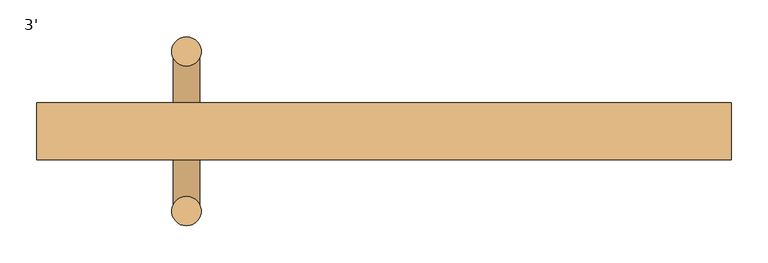
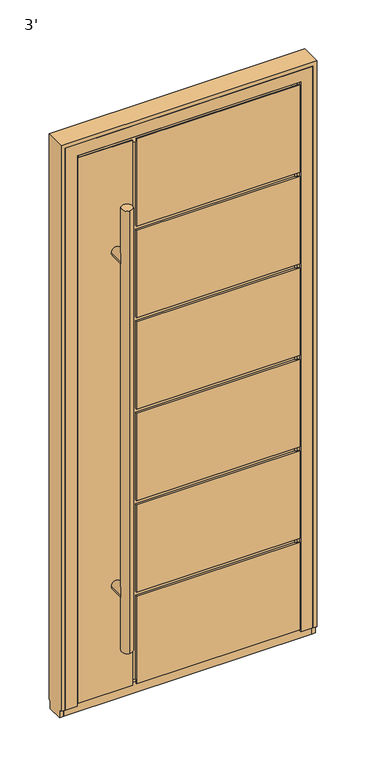
"""IFC4 building model written with IfcOpenShell, lengths in millimetres: door geometry, 3'."""

from ifc_helpers import new_model, si_unit, point, frame, frame_2d, origin, place, context, project, spatial, circle_curve, trimmed, segment, composite_curve, outline, extrude, faceted_brep, source, transform, mapped, element, save


def door_3_79df91aa(model_context):
    return source(origin(), model_context, "Body", "SolidModel", [
        extrude(outline(composite_curve([segment(trimmed(circle_curve(frame_2d((-268.65, 90.8003001)), 20.0), [point((-268.65, 70.8003001))], [point((-268.65, 110.8003001))], False, "CARTESIAN"), True, "CONTINUOUS"), segment(trimmed(circle_curve(frame_2d((-268.65, 90.8003001)), 20.0), [point((-268.65, 110.8003001))], [point((-268.65, 70.8003001))], False, "CARTESIAN"), True, "CONTINUOUS")], self_intersect=False)), frame((0.0, 0.0, 210.0000003), z_axis=(0.0, 0.0, 1.0), x_axis=(1.0, 0.0, 0.0)), (0.0, 0.0, 1.0), 1724.5),
        extrude(outline(composite_curve([segment(trimmed(circle_curve(frame_2d((-268.65, -126.2003001)), 20.0), [point((-268.65, -146.2003001))], [point((-268.65, -106.2003001))], False, "CARTESIAN"), True, "CONTINUOUS"), segment(trimmed(circle_curve(frame_2d((-268.65, -126.2003001)), 20.0), [point((-268.65, -106.2003001))], [point((-268.65, -146.2003001))], False, "CARTESIAN"), True, "CONTINUOUS")], self_intersect=False)), frame((0.0, 0.0, 210.0000003), z_axis=(0.0, 0.0, 1.0), x_axis=(1.0, 0.0, 0.0)), (0.0, 0.0, 1.0), 1724.5),
        extrude(outline(composite_curve([segment(trimmed(circle_curve(frame_2d((422.2500003, -268.65)), 18.0), [point((422.2500003, -286.65))], [point((422.2500003, -250.65))], False, "CARTESIAN"), True, "CONTINUOUS"), segment(trimmed(circle_curve(frame_2d((422.2500003, -268.65)), 18.0), [point((422.2500003, -250.65))], [point((422.2500003, -286.65))], False, "CARTESIAN"), True, "CONTINUOUS")], self_intersect=False)), frame((0.0, -126.2, 0.0), z_axis=(0.0, 1.0, 0.0), x_axis=(0.0, 0.0, 1.0)), (0.0, 0.0, 1.0), 217.0),
        extrude(outline(composite_curve([segment(trimmed(circle_curve(frame_2d((1722.2500003, -268.65)), 18.0), [point((1722.2500003, -286.65))], [point((1722.2500003, -250.65))], False, "CARTESIAN"), True, "CONTINUOUS"), segment(trimmed(circle_curve(frame_2d((1722.2500003, -268.65)), 18.0), [point((1722.2500003, -250.65))], [point((1722.2500003, -286.65))], False, "CARTESIAN"), True, "CONTINUOUS")], self_intersect=False)), frame((0.0, -126.2, 0.0), z_axis=(0.0, 1.0, 0.0), x_axis=(0.0, 0.0, 1.0)), (0.0, 0.0, 1.0), 217.0),
        faceted_brep([(-193.65, 13.8, 366.5833337), (383.65, 13.8, 366.5833337), (383.65, 13.8, 351.5833337), (-193.65, 13.8, 351.5833337), (-193.65, 13.8, 35.0), (-208.65, 13.8, 35.0), (-208.65, 13.8, 2109.5000003), (-193.65, 13.8, 2109.5000003), (-193.65, 13.8, 1792.916667), (383.65, 13.8, 1792.916667), (383.65, 13.8, 1777.916667), (-193.65, 13.8, 1777.916667), (-193.65, 13.8, 1436.3333337), (383.65, 13.8, 1436.3333337), (383.65, 13.8, 1421.3333337), (-193.65, 13.8, 1421.3333337), (-193.65, 13.8, 1079.7500004), (383.65, 13.8, 1079.7500004), (383.65, 13.8, 1064.7500004), (-193.65, 13.8, 1064.7500004), (-193.65, 13.8, 723.166667), (383.65, 13.8, 723.166667), (383.65, 13.8, 708.166667), (-193.65, 13.8, 708.166667), (-193.65, 20.8, 708.166667), (-193.65, 20.8, 366.5833337), (383.65, 20.8, 708.166667), (383.65, 11.7997698, 2109.5000003), (383.65, 11.7997698, 35.0), (383.65, 18.8020472, 35.0), (383.65, 18.8020472, 24.0), (383.65, 20.8, 24.0), (383.65, 20.8, 351.5833337), (383.65, 20.8, 366.5833337), (383.65, 20.8, 723.166667), (383.65, 20.8, 1064.7500004), (383.65, 20.8, 1079.7500004), (383.65, 20.8, 1421.3333337), (383.65, 20.8, 1436.3333337), (383.65, 20.8, 1777.916667), (383.65, 20.8, 1792.916667), (383.65, 20.8, 2109.5000003), (-193.65, 20.8, 723.166667), (-193.65, 20.8, 1064.7500004), (-193.65, 20.8, 1079.7500004), (-193.65, 20.8, 1421.3333337), (-208.65, 18.8020472, 35.0), (-208.65, 18.8020472, 24.0), (-208.65, 20.8, 24.0), (-208.65, 20.8, 2109.5000003), (-383.65, 11.7997698, 35.0), (-383.65, 18.8020472, 35.0), (-193.65, 18.8020472, 35.0), (-193.65, 20.8, 351.5833337), (-193.65, 20.8, 24.0), (-193.65, 18.8020472, 24.0), (-383.65, 18.8020472, 24.0), (-383.65, 20.8, 24.0), (-383.65, 20.8, 2109.5000003), (-193.65, 20.8, 1436.3333337), (-193.65, 20.8, 1777.916667), (-193.65, 20.8, 1792.916667), (-193.65, 20.8, 2109.5000003), (408.65, -56.2, 10.0000003), (-193.65, -56.2, 10.0000003), (-193.65, -53.2, 10.0000003), (408.65, -53.2, 10.0000003), (-408.65, -53.2, 10.0000003), (-208.65, -53.2, 10.0000003), (-208.65, -56.2, 10.0000003), (-408.65, -56.2, 10.0000003), (408.65, -56.2, 366.5833337), (408.65, -53.2, 366.5833337), (408.65, -53.2, 708.166667), (408.65, -56.2, 708.166667), (408.65, -56.2, 1079.7500004), (408.65, -53.2, 1079.7500004), (408.65, -53.2, 1421.3333337), (408.65, -56.2, 1421.3333337), (408.65, -56.2, 723.166667), (408.65, -53.2, 723.166667), (408.65, -53.2, 1064.7500004), (408.65, -56.2, 1064.7500004), (408.65, -56.2, 1436.3333337), (408.65, -53.2, 1436.3333337), (408.65, -53.2, 1777.916667), (408.65, -56.2, 1777.916667), (408.65, -56.2, 2134.5000003), (408.65, -56.2, 1792.916667), (408.65, -53.2, 1792.916667), (408.65, -53.2, 2134.5000003), (408.65, -53.2, 351.5833337), (408.65, -56.2, 351.5833337), (-193.65, -53.2, 25.5), (393.15, -53.2, 25.5), (393.15, -53.2, 351.5833337), (393.15, -53.2, 366.5833337), (393.15, -53.2, 708.166667), (393.15, -53.2, 1079.7500004), (393.15, -53.2, 1421.3333337), (393.15, -53.2, 723.166667), (393.15, -53.2, 1064.7500004), (-393.15, -53.2, 25.5), (-208.65, -53.2, 25.5), (-408.65, -53.2, 2134.5000003), (-208.65, -53.2, 2134.5000003), (-208.65, -53.2, 2119.0000003), (-393.15, -53.2, 2119.0000003), (393.15, -53.2, 1436.3333337), (393.15, -53.2, 1777.916667), (393.15, -53.2, 1792.916667), (393.15, -53.2, 2119.0000003), (-193.65, -53.2, 2119.0000003), (-193.65, -53.2, 2134.5000003), (-193.65, -49.2, 351.5833337), (-193.65, -49.2, 25.5), (-193.65, -56.2, 351.5833337), (-208.65, -56.2, 2134.5000003), (-408.65, -56.2, 2134.5000003), (-193.65, -56.2, 708.166667), (-193.65, -56.2, 366.5833337), (-193.65, -56.2, 1421.3333337), (-193.65, -56.2, 1079.7500004), (-193.65, -56.2, 1064.7500004), (-193.65, -56.2, 723.166667), (-193.65, -56.2, 1777.916667), (-193.65, -56.2, 1436.3333337), (-193.65, -56.2, 2134.5000003), (-193.65, -56.2, 1792.916667), (-208.65, -49.2, 2119.0000003), (-208.65, -49.2, 25.5), (-383.65, 11.7997698, 2109.5000003), (393.15, 11.7997698, 2119.0000003), (393.15, 11.7997698, 25.5), (-393.15, 11.7997698, 25.5), (-393.15, 11.7997698, 2119.0000003), (393.15, -49.2, 1792.916667), (393.15, -49.2, 1777.916667), (393.15, -49.2, 1436.3333337), (393.15, -49.2, 1421.3333337), (393.15, -49.2, 1079.7500004), (393.15, -49.2, 1064.7500004), (393.15, -49.2, 723.166667), (393.15, -49.2, 708.166667), (393.15, -49.2, 366.5833337), (393.15, -49.2, 351.5833337), (-193.65, -49.2, 1777.916667), (-193.65, -49.2, 1792.916667), (-193.65, -49.2, 2119.0000003), (-193.65, -49.2, 366.5833337), (-193.65, -49.2, 708.166667), (-193.65, -49.2, 723.166667), (-193.65, -49.2, 1064.7500004), (-193.65, -49.2, 1079.7500004), (-193.65, -49.2, 1421.3333337), (-193.65, -49.2, 1436.3333337)], [[[0, 1, 2, 3, 4, 5, 6, 7, 8, 9, 10, 11, 12, 13, 14, 15, 16, 17, 18, 19, 20, 21, 22, 23]], [[23, 24, 25, 0]], [[23, 22, 26, 24]], [[27, 28, 29, 30, 31, 32, 2, 1, 33, 26, 22, 21, 34, 35, 18, 17, 36, 37, 14, 13, 38, 39, 10, 9, 40, 41]], [[42, 34, 21, 20]], [[19, 43, 42, 20]], [[19, 18, 35, 43]], [[44, 36, 17, 16]], [[15, 45, 44, 16]], [[5, 46, 47, 48, 49, 6]], [[28, 50, 51, 46, 5, 4, 52, 29]], [[53, 54, 55, 52, 4, 3]], [[3, 2, 32, 53]], [[25, 33, 1, 0]], [[29, 52, 55, 30]], [[56, 47, 46, 51]], [[30, 55, 54, 31]], [[57, 48, 47, 56]], [[36, 44, 45, 37]], [[34, 42, 43, 35]], [[33, 25, 24, 26]], [[54, 53, 32, 31]], [[58, 49, 48, 57]], [[38, 59, 60, 39]], [[41, 40, 61, 62]], [[63, 64, 65, 66]], [[67, 68, 69, 70]], [[71, 72, 73, 74]], [[75, 76, 77, 78]], [[79, 80, 81, 82]], [[83, 84, 85, 86]], [[87, 88, 89, 90]], [[66, 91, 92, 63]], [[65, 93, 94, 95, 91, 66]], [[72, 96, 97, 73]], [[76, 98, 99, 77]], [[80, 100, 101, 81]], [[102, 103, 68, 67, 104, 105, 106, 107]], [[84, 108, 109, 85]], [[90, 89, 110, 111, 112, 113]], [[114, 115, 93, 65, 64, 116]], [[70, 69, 117, 118]], [[63, 92, 116, 64]], [[74, 119, 120, 71]], [[78, 121, 122, 75]], [[82, 123, 124, 79]], [[86, 125, 126, 83]], [[87, 127, 128, 88]], [[70, 118, 104, 67]], [[129, 106, 105, 117, 69, 68, 103, 130]], [[58, 57, 56, 51, 50, 131]], [[132, 133, 134, 135], [131, 50, 28, 27]], [[111, 110, 136, 137, 109, 108, 138, 139, 99, 98, 140, 141, 101, 100, 142, 143, 97, 96, 144, 145, 95, 94, 133, 132]], [[94, 93, 115, 130, 103, 102, 134, 133]], [[135, 134, 102, 107]], [[146, 137, 136, 147, 148, 129, 130, 115, 114, 145, 144, 149, 150, 143, 142, 151, 152, 141, 140, 153, 154, 139, 138, 155]], [[153, 122, 121, 154]], [[153, 140, 98, 76, 75, 122]], [[123, 82, 81, 101, 141, 152]], [[151, 124, 123, 152]], [[151, 142, 100, 80, 79, 124]], [[119, 74, 73, 97, 143, 150]], [[149, 120, 119, 150]], [[149, 144, 96, 72, 71, 120]], [[116, 92, 91, 95, 145, 114]], [[15, 14, 37, 45]], [[59, 38, 13, 12]], [[11, 60, 59, 12]], [[11, 10, 39, 60]], [[61, 40, 9, 8]], [[8, 7, 62, 61]], [[125, 86, 85, 109, 137, 146]], [[128, 127, 113, 112, 148, 147]], [[121, 78, 77, 99, 139, 154]], [[155, 138, 108, 84, 83, 126]], [[155, 126, 125, 146]], [[147, 136, 110, 89, 88, 128]], [[90, 113, 127, 87]], [[118, 117, 105, 104]], [[132, 135, 107, 106, 129, 148, 112, 111]], [[27, 41, 62, 7, 6, 49, 58, 131]]]),
        faceted_brep([(-457.2, -56.2, 0.0), (-457.2, -47.1997571, 0.0), (-412.7, -47.1997571, 0.0), (-412.7, -56.2, 0.0), (-403.2, 16.2999958, 0.0), (-403.2, 11.8, 0.0), (-457.2, 11.8, 0.0), (-457.2, 20.8, 0.0), (-387.7, 20.8, 0.0), (-387.7, 16.2999958, 0.0), (457.2, 20.8, 0.0), (457.2, 11.8, 0.0), (403.2, 11.8, 0.0), (403.2, 16.2999958, 0.0), (387.7, 16.2999958, 0.0), (387.7, 20.8, 0.0), (412.7, -47.1997571, 0.0), (457.2, -47.1997571, 0.0), (457.2, -56.2, 0.0), (412.7, -56.2, 0.0), (-457.2, 11.8, -30.0), (-457.2, -47.1997571, -30.0), (-457.2, -56.2, 2189.5), (-457.2, 20.8, 2189.5), (-412.7, -56.2, 2145.0), (412.7, -56.2, 2145.0), (457.2, -56.2, 2189.5), (457.2, 20.8, 2189.5), (457.2, -47.1997571, -30.0), (457.2, 11.8, -30.0), (387.7, 20.8, 2120.0), (-387.7, 20.8, 2120.0), (-403.2, -47.2, 2135.5), (-403.2, -47.2, 14.5), (-403.2, 11.8, 14.5), (-403.2, 16.2999958, 2135.5), (403.2, 16.2999958, 2135.5), (403.2, -47.2, 2135.5), (403.2, 11.8, 14.5), (403.2, -47.2, 14.5), (-412.7, -47.2, 2145.0), (412.7, -47.2, 2145.0), (-387.7, 16.2999958, 2120.0), (387.7, 16.2999958, 2120.0)], [[[0, 1, 2, 3]], [[4, 5, 6, 7, 8, 9]], [[10, 11, 12, 13, 14, 15]], [[16, 17, 18, 19]], [[7, 6, 20, 21, 1, 0, 22, 23]], [[3, 24, 25, 19, 18, 26, 22, 0]], [[22, 26, 27, 23]], [[18, 17, 28, 29, 11, 10, 27, 26]], [[7, 23, 27, 10, 15, 30, 31, 8]], [[32, 33, 34, 5, 4, 35]], [[35, 36, 37, 32]], [[36, 13, 12, 38, 39, 37]], [[40, 24, 3, 2]], [[16, 41, 40, 2, 1, 21, 28, 17], [37, 39, 33, 32]], [[9, 42, 43, 14, 13, 36, 35, 4]], [[8, 31, 42, 9]], [[24, 40, 41, 25]], [[30, 43, 42, 31]], [[19, 25, 41, 16]], [[14, 43, 30, 15]], [[20, 6, 5, 34, 38, 12, 11, 29]], [[39, 38, 34, 33]], [[20, 29, 28, 21]]]),
        faceted_brep([(-457.2, -47.2, -30.0), (-472.2, -47.2, -30.0), (-472.2, 11.8, -30.0), (-457.2, 11.8, -30.0), (-457.2, -56.2, 2189.5), (-457.2, -56.2, 0.0), (-457.2, -47.2, 0.0), (-457.2, 11.8, 0.0), (-457.2, 20.8, 0.0), (-457.2, 20.8, 2189.5), (-472.2, 11.8, 0.0), (472.2, 11.8, 0.0), (472.2, 11.8, -30.0), (457.2, 11.8, -30.0), (457.2, 11.8, 0.0), (-472.2, 20.8, 2204.5), (-472.2, 20.8, 0.0), (-472.2, -47.2, 0.0), (-472.2, -56.2, 0.0), (-472.2, -56.2, 2204.5), (457.2, -47.2, 0.0), (457.2, -47.2, -30.0), (472.2, -47.2, -30.0), (472.2, -47.2, 0.0), (457.2, 20.8, 2189.5), (457.2, 20.8, 0.0), (457.2, -56.2, 0.0), (457.2, -56.2, 2189.5), (472.2, -56.2, 0.0), (472.2, -56.2, 2204.5), (472.2, 20.8, 0.0), (472.2, 20.8, 2204.5)], [[[0, 1, 2, 3]], [[4, 5, 6, 0, 3, 7, 8, 9]], [[7, 3, 2, 10]], [[11, 12, 13, 14]], [[15, 16, 10, 2, 1, 17, 18, 19]], [[17, 1, 0, 6]], [[20, 21, 22, 23]], [[24, 25, 14, 13, 21, 20, 26, 27]], [[27, 26, 28, 29, 19, 18, 5, 4]], [[6, 5, 18, 17]], [[23, 28, 26, 20]], [[22, 21, 13, 12]], [[10, 16, 8, 7]], [[14, 25, 30, 11]], [[9, 8, 16, 15, 31, 30, 25, 24]], [[29, 28, 23, 22, 12, 11, 30, 31]], [[9, 24, 27, 4]], [[19, 29, 31, 15]]]),
    ])


if __name__ == "__main__":
    model = new_model("IFC4")
    model_context = context("Model", 3, world=origin())
    ifc_project = project(units=[si_unit("LENGTHUNIT", "METRE", prefix="MILLI")], contexts=[model_context])
    site = spatial("IfcSite", under=ifc_project)
    building = spatial("IfcBuilding", under=site)
    placement = place(None, origin())
    door_3_shape = door_3_79df91aa(model_context)
    element("IfcDoor", 1, ObjectType="3'", at=placement, inside=building, context=model_context, shape_type="MappedRepresentation", body=[
        mapped(door_3_shape, transform((0.0, 0.0, 0.0), x_axis=(1.0, 0.0, 0.0), y_axis=(0.0, 1.0, 0.0), z_axis=(0.0, 0.0, 1.0))),
    ])
    save(model, "model.ifc")

# Revit data of these elements
# Type "3'"
#   Type Mark = "15"
#   Water resistance = "up to Class E900, EN 12208:2001"
#   Uniclass2015Version = "v1.21"
#   Uniclass2015Reference = "Ss_25_30_20_30"
#   Uniclass2015Description = "Frame and door leaf system"
#   URL = "www.aluprof.com"
#   Type IFC Predefined Type = "USERDEFINED"
#   Right-hand / Left-hand door [instance default] = ""
#   Resistance to wind load = "up to Class C5/B5, EN 12210:2001"
#   Insert type = "ST"
#   Hardware [instance default] = ""
#   Product page = "https://aluprof.com/en/architects/offer/window-and-door-systems/panel-doors#visualisation"
#   Operation = "SinglePanelOutwardOpening"
#   Opening type = "Outward"
#   NBSReference = "25-50-20/125"
#   NBSDescription = "Frame and door leaf system"
#   Important = "The actual acceptable construction dimensions are dependent on the selection of profiles and hardware, glazing type, construction weight and the construction’s operating conditions. These should be determined by a suitably qualified person, and using ALUPROF’s calculation software"
#   IfcExportType = "USERDEFINED"
#   IfcExportAs = "IfcDoorType"
#   Handle type [instance default] = ""
#   Manufacturer = "ALUPROF SA"
#   Export Type to IFC As = "IfcDoorType"
#   Door sill type [instance default] = ""
#   Description = "External single-leaf panel door outward opening"
#   Model = "MB-86 ST Panel Door AD07"
#   Content of the recyclate in the material = "69.2%"
#   COBie.Type.WarrantyDurationParts = ""
#   COBie.Type.Name = ""
#   COBie.Type.Manufacturer = "ALUPROF SA"
#   COBie.Space.Name = ""
#   COBie.Floor.Name = ""
#   COBie.Facility.Name = ""
#   COBie.CreatedOn = ""
#   COBie.Component.WarrantyStartDate = ""
#   COBie.Component.Name = "MB-86 ST Panel Door AD07"
#   Burglar resistance = "RC2"
#   Air permeability = "up to Class 4, EN 12207:2001"
#   Width of the active leaf = 2' - 8.17717"
#   Placement in wall = 0' - 0.7874"
#   Thickness = 0' - 3.0315"
#   Height of the opening sash = 6' - 11.64173"
#   Handle Offset = 3' - 5.33858"
#   Rough Height = 7' - 4.61024"
#   Rough Width = 3' - 1.1811"
#   Height = 7' - 2.20079"
#   Width = 3' - 0"
#   Construction depth = 0' - 3.0315"
#   Clear opening width = 2' - 3.94882"
#   Clear opening height = 6' - 10.67717"
#   Height of the array = 1' - 1.44816"
#   Schedule No. [instance default] = 1
#   Handrail [instance default] = yes
#   IsExternal = yes
#   Handle [instance default] = no
#   Door closer [instance default] = no
#   Function = 1
#   COBie.Type = yes
#   COBie = yes
#   Access control [instance default] = no
#   Panel = element 387710
#   Wall Closure = (empty or 0)
